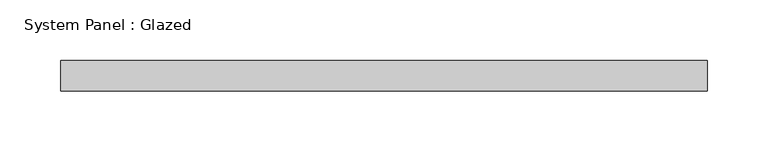
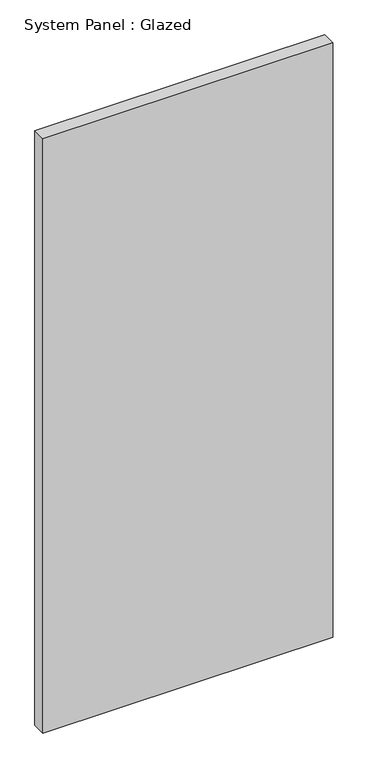
"""IFC4 building model written with IfcOpenShell, lengths in millimetres: plate geometry, System Panel : Glazed."""

from ifc_helpers import new_model, si_unit, origin, origin_with_axes, place, context, project, spatial, polyline, outline, extrude, source, transform, mapped, element, save


def system_panel_glazed_8f98839e(model_context):
    return source(origin(), model_context, "Body", "SweptSolid", [
        extrude(outline(polyline([(266.7, 19.05), (-266.7, 19.05), (-266.7, 44.45), (266.7, 44.45), (266.7, 19.05)])), origin_with_axes(), (0.0, 0.0, 1.0), 1155.7),
    ])


if __name__ == "__main__":
    model = new_model("IFC4")
    model_context = context("Model", 3, world=origin())
    ifc_project = project(units=[si_unit("LENGTHUNIT", "METRE", prefix="MILLI")], contexts=[model_context])
    site = spatial("IfcSite", under=ifc_project)
    building = spatial("IfcBuilding", under=site)
    placement = place(None, origin())
    system_panel_glazed_shape = system_panel_glazed_8f98839e(model_context)
    element("IfcPlate", 1, ObjectType="System Panel : Glazed", at=placement, inside=building, context=model_context, shape_type="MappedRepresentation", body=[
        mapped(system_panel_glazed_shape, transform((0.0, 0.0, 0.0), x_axis=(1.0, 0.0, 0.0), y_axis=(0.0, 1.0, 0.0), z_axis=(0.0, 0.0, 1.0))),
    ])
    save(model, "model.ifc")

# Revit data of these elements
# Type "System Panel : Glazed"
#   Construction Type Id = "GSP4R"
#   Analytic Construction = "1/8 in Pilkington single glazing"
#   Visual Light Transmittance = 0.9
#   Solar Heat Gain Coefficient = 0.86
#   Heat Transfer Coefficient (U) = 1.18115 BTU/(h·ft²·°F)
# Element 1 (IfcPlate, "System Panel : Glazed")
#   Materials on its faces: "Glass"
# Materials
#   "Glass": class "Glass", colour RGB 0 128 192, transparency 0.75, Description = "Soda Lime Glass", Cost = 0
